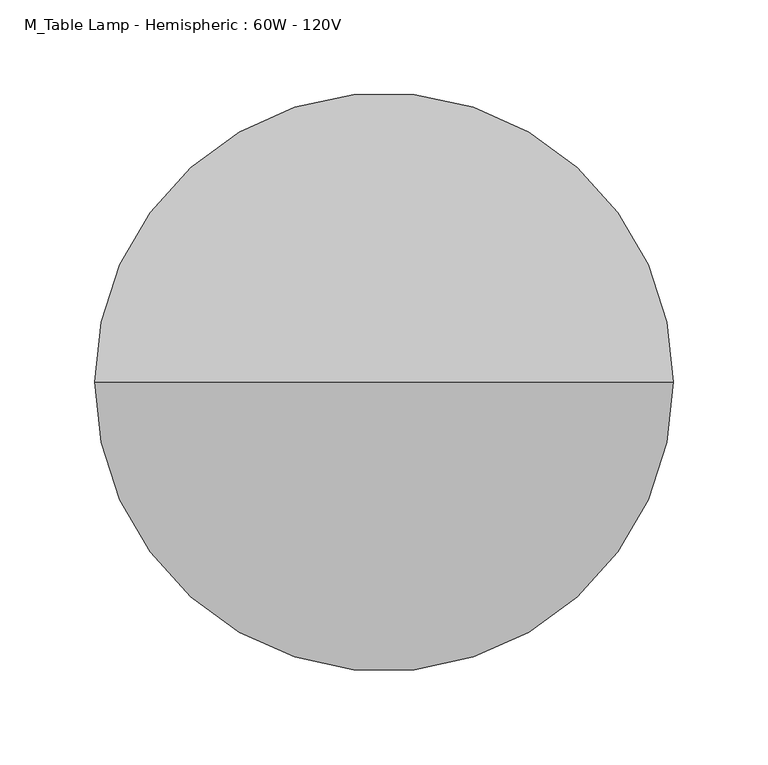
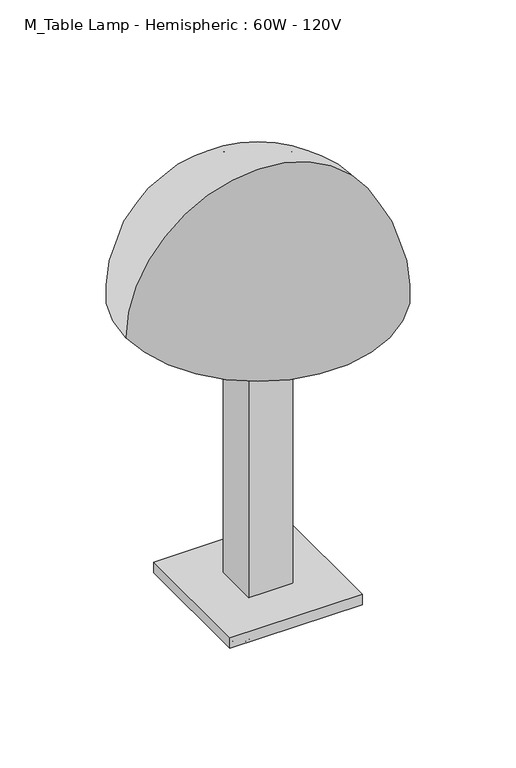
"""IFC4 building model written with IfcOpenShell, lengths in millimetres: light fixture geometry, M_Table Lamp - Hemispheric : 60W - 120V."""

from ifc_helpers import new_model, si_unit, point, frame, origin, origin_2d, place, context, project, spatial, polyline, circle_curve, ellipse_curve, trimmed, segment, composite_curve, outline, extrude, source, transform, mapped, element, save
from ifc_brep_helpers import plane_surface, revolved_surface, advanced_brep


def m_table_lamp_hemispheric_60w_120v_fef6e77c(model_context):
    return source(origin(), model_context, "Body", "SolidModel", [
        extrude(outline(polyline([(76.2, 76.2), (76.2, -76.2), (-76.2, -76.2), (-76.2, 76.2), (76.2, 76.2)])), frame((0.0, 0.0, 12.7), z_axis=(0.0, 0.0, 1.0), x_axis=(1.0, 0.0, 0.0)), (0.0, 0.0, 1.0), 12.7),
        advanced_brep(
        [(34.925, 50.8, 12.7), (66.675, 50.8, 12.7), (53.975, 50.8, 0.0), (47.625, 50.8, 0.0), (47.625, 50.8, 12.7), (53.975, 50.8, 12.7)],
        [
            (0, 1, circle_curve(frame((50.8, 50.8, 12.7), z_axis=(0.0, 0.0, -1.0), x_axis=(1.0, 0.0, 0.0)), 15.875)),
            (1, 2, circle_curve(frame((53.975, 50.8, 12.7), z_axis=(0.0, 1.0, 0.0), x_axis=(1.0, 0.0, 0.0)), 12.7)),
            (2, 3, circle_curve(frame((50.8, 50.8, 0.0), z_axis=(0.0, 0.0, 1.0), x_axis=(1.0, 0.0, 0.0)), 3.175)),
            (3, 0, circle_curve(frame((47.625, 50.8, 12.7), z_axis=(0.0, 1.0, 0.0), x_axis=(-1.0, 0.0, 0.0)), 12.7)),
            (1, 0, circle_curve(frame((50.8, 50.8, 12.7), z_axis=(0.0, 0.0, -1.0), x_axis=(1.0, 0.0, 0.0)), 15.875)),
            (3, 2, circle_curve(frame((50.8, 50.8, 0.0), z_axis=(0.0, 0.0, 1.0), x_axis=(1.0, 0.0, 0.0)), 3.175)),
            (4, 5, circle_curve(frame((50.8, 50.8, 12.7), z_axis=(0.0, 0.0, -1.0), x_axis=(1.0, 0.0, 0.0)), 3.175)),
            (5, 1),
            (0, 4),
            (5, 4, circle_curve(frame((50.8, 50.8, 12.7), z_axis=(0.0, 0.0, -1.0), x_axis=(1.0, 0.0, 0.0)), 3.175)),
            (2, 5),
            (4, 3),
        ],
        [
            revolved_surface(trimmed(ellipse_curve(frame((53.975, 50.8, 12.7), z_axis=(0.0, -1.0, 0.0), x_axis=(1.0, 0.0, 0.0)), 12.7, 12.7), [point((53.975, 50.8, 0.0))], [point((66.675, 50.8, 12.7))], True, "CARTESIAN"), (50.8, 50.8, 36.0623287), (0.0, 0.0, 1.0)),
            plane_surface(frame((50.8, 50.8, 12.7), z_axis=(0.0, 0.0, 1.0), x_axis=(1.0, 0.0, 0.0))),
            revolved_surface(polyline([(53.974999999999994, 50.8, 12.7), (53.974999999999994, 50.8, 0.0)]), (50.8, 50.8, 36.0623287), (0.0, 0.0, 1.0)),
        ],
        [
            (0, [[1, 2, 3, 4]]),
            (0, [[5, -4, 6, -2]]),
            (1, [[7, 8, -1, 9]]),
            (1, [[10, -9, -5, -8]]),
            (2, [[-3, 11, -7, 12]]),
            (2, [[-6, -12, -10, -11]]),
        ],
    ),
        advanced_brep(
        [(34.9494337, -50.8, 12.7), (66.6994337, -50.8, 12.7), (53.9994337, -50.8, 0.0), (47.6494337, -50.8, 0.0), (47.6494337, -50.8, 12.7), (53.9994337, -50.8, 12.7)],
        [
            (0, 1, circle_curve(frame((50.8244337, -50.8, 12.7), z_axis=(0.0, 0.0, -1.0), x_axis=(1.0, 0.0, 0.0)), 15.875)),
            (1, 2, circle_curve(frame((53.9994337, -50.8, 12.7), z_axis=(0.0, 1.0, 0.0), x_axis=(1.0, 0.0, 0.0)), 12.7)),
            (2, 3, circle_curve(frame((50.8244337, -50.8, 0.0), z_axis=(0.0, 0.0, 1.0), x_axis=(1.0, 0.0, 0.0)), 3.175)),
            (3, 0, circle_curve(frame((47.6494337, -50.8, 12.7), z_axis=(0.0, 1.0, 0.0), x_axis=(-1.0, 0.0, 0.0)), 12.7)),
            (1, 0, circle_curve(frame((50.8244337, -50.8, 12.7), z_axis=(0.0, 0.0, -1.0), x_axis=(1.0, 0.0, 0.0)), 15.875)),
            (3, 2, circle_curve(frame((50.8244337, -50.8, 0.0), z_axis=(0.0, 0.0, 1.0), x_axis=(1.0, 0.0, 0.0)), 3.175)),
            (4, 5, circle_curve(frame((50.8244337, -50.8, 12.7), z_axis=(0.0, 0.0, -1.0), x_axis=(1.0, 0.0, 0.0)), 3.175)),
            (5, 1),
            (0, 4),
            (5, 4, circle_curve(frame((50.8244337, -50.8, 12.7), z_axis=(0.0, 0.0, -1.0), x_axis=(1.0, 0.0, 0.0)), 3.175)),
            (2, 5),
            (4, 3),
        ],
        [
            revolved_surface(trimmed(ellipse_curve(frame((53.9994337, -50.8, 12.7), z_axis=(0.0, -1.0, 0.0), x_axis=(1.0, 0.0, 0.0)), 12.7, 12.7), [point((53.9994337, -50.8, 0.0))], [point((66.6994337, -50.8, 12.7))], True, "CARTESIAN"), (50.8244337, -50.8, 36.0623287), (0.0, 0.0, 1.0)),
            plane_surface(frame((50.8244337, -50.8, 12.7), z_axis=(0.0, 0.0, 1.0), x_axis=(1.0, 0.0, 0.0))),
            revolved_surface(polyline([(53.9994337, -50.8, 12.7), (53.9994337, -50.8, 0.0)]), (50.8244337, -50.8, 36.0623287), (0.0, 0.0, 1.0)),
        ],
        [
            (0, [[1, 2, 3, 4]]),
            (0, [[5, -4, 6, -2]]),
            (1, [[7, 8, -1, 9]]),
            (1, [[10, -9, -5, -8]]),
            (2, [[-3, 11, -7, 12]]),
            (2, [[-6, -12, -10, -11]]),
        ],
    ),
        advanced_brep(
        [(-66.7581301, 50.8, 12.7), (-35.0081301, 50.8, 12.7), (-47.7081301, 50.8, 0.0), (-54.0581301, 50.8, 0.0), (-54.0581301, 50.8, 12.7), (-47.7081301, 50.8, 12.7)],
        [
            (0, 1, circle_curve(frame((-50.8831301, 50.8, 12.7), z_axis=(0.0, 0.0, -1.0), x_axis=(1.0, 0.0, 0.0)), 15.875)),
            (1, 2, circle_curve(frame((-47.7081301, 50.8, 12.7), z_axis=(0.0, 1.0, 0.0), x_axis=(1.0, 0.0, 0.0)), 12.7)),
            (2, 3, circle_curve(frame((-50.8831301, 50.8, 0.0), z_axis=(0.0, 0.0, 1.0), x_axis=(1.0, 0.0, 0.0)), 3.175)),
            (3, 0, circle_curve(frame((-54.0581301, 50.8, 12.7), z_axis=(0.0, 1.0, 0.0), x_axis=(-1.0, 0.0, 0.0)), 12.7)),
            (1, 0, circle_curve(frame((-50.8831301, 50.8, 12.7), z_axis=(0.0, 0.0, -1.0), x_axis=(1.0, 0.0, 0.0)), 15.875)),
            (3, 2, circle_curve(frame((-50.8831301, 50.8, 0.0), z_axis=(0.0, 0.0, 1.0), x_axis=(1.0, 0.0, 0.0)), 3.175)),
            (4, 5, circle_curve(frame((-50.8831301, 50.8, 12.7), z_axis=(0.0, 0.0, -1.0), x_axis=(1.0, 0.0, 0.0)), 3.175)),
            (5, 1),
            (0, 4),
            (5, 4, circle_curve(frame((-50.8831301, 50.8, 12.7), z_axis=(0.0, 0.0, -1.0), x_axis=(1.0, 0.0, 0.0)), 3.175)),
            (2, 5),
            (4, 3),
        ],
        [
            revolved_surface(trimmed(ellipse_curve(frame((-47.7081301, 50.8, 12.7), z_axis=(0.0, -1.0, 0.0), x_axis=(1.0, 0.0, 0.0)), 12.7, 12.7), [point((-47.7081301, 50.8, 0.0))], [point((-35.0081301, 50.8, 12.7))], True, "CARTESIAN"), (-50.8831301, 50.8, 36.0623287), (0.0, 0.0, 1.0)),
            plane_surface(frame((-50.8831301, 50.8, 12.7), z_axis=(0.0, 0.0, 1.0), x_axis=(1.0, 0.0, 0.0))),
            revolved_surface(polyline([(-47.708130100000005, 50.8, 12.7), (-47.708130100000005, 50.8, 0.0)]), (-50.8831301, 50.8, 36.0623287), (0.0, 0.0, 1.0)),
        ],
        [
            (0, [[1, 2, 3, 4]]),
            (0, [[5, -4, 6, -2]]),
            (1, [[7, 8, -1, 9]]),
            (1, [[10, -9, -5, -8]]),
            (2, [[-3, 11, -7, 12]]),
            (2, [[-6, -12, -10, -11]]),
        ],
    ),
        advanced_brep(
        [(-66.7336963, -50.8, 12.7), (-34.9836963, -50.8, 12.7), (-47.6836963, -50.8, 0.0), (-54.0336963, -50.8, 0.0), (-54.0336963, -50.8, 12.7), (-47.6836963, -50.8, 12.7)],
        [
            (0, 1, circle_curve(frame((-50.8586963, -50.8, 12.7), z_axis=(0.0, 0.0, -1.0), x_axis=(1.0, 0.0, 0.0)), 15.875)),
            (1, 2, circle_curve(frame((-47.6836963, -50.8, 12.7), z_axis=(0.0, 1.0, 0.0), x_axis=(1.0, 0.0, 0.0)), 12.7)),
            (2, 3, circle_curve(frame((-50.8586963, -50.8, 0.0), z_axis=(0.0, 0.0, 1.0), x_axis=(1.0, 0.0, 0.0)), 3.175)),
            (3, 0, circle_curve(frame((-54.0336963, -50.8, 12.7), z_axis=(0.0, 1.0, 0.0), x_axis=(-1.0, 0.0, 0.0)), 12.7)),
            (1, 0, circle_curve(frame((-50.8586963, -50.8, 12.7), z_axis=(0.0, 0.0, -1.0), x_axis=(1.0, 0.0, 0.0)), 15.875)),
            (3, 2, circle_curve(frame((-50.8586963, -50.8, 0.0), z_axis=(0.0, 0.0, 1.0), x_axis=(1.0, 0.0, 0.0)), 3.175)),
            (4, 5, circle_curve(frame((-50.8586963, -50.8, 12.7), z_axis=(0.0, 0.0, -1.0), x_axis=(1.0, 0.0, 0.0)), 3.175)),
            (5, 1),
            (0, 4),
            (5, 4, circle_curve(frame((-50.8586963, -50.8, 12.7), z_axis=(0.0, 0.0, -1.0), x_axis=(1.0, 0.0, 0.0)), 3.175)),
            (2, 5),
            (4, 3),
        ],
        [
            revolved_surface(trimmed(ellipse_curve(frame((-47.6836963, -50.8, 12.7), z_axis=(0.0, -1.0, 0.0), x_axis=(1.0, 0.0, 0.0)), 12.7, 12.7), [point((-47.6836963, -50.8, 0.0))], [point((-34.9836963, -50.8, 12.7))], True, "CARTESIAN"), (-50.8586963, -50.8, 36.0623287), (0.0, 0.0, 1.0)),
            plane_surface(frame((-50.8586963, -50.8, 12.7), z_axis=(0.0, 0.0, 1.0), x_axis=(1.0, 0.0, 0.0))),
            revolved_surface(polyline([(-47.6836963, -50.8, 12.7), (-47.6836963, -50.8, 0.0)]), (-50.8586963, -50.8, 36.0623287), (0.0, 0.0, 1.0)),
        ],
        [
            (0, [[1, 2, 3, 4]]),
            (0, [[5, -4, 6, -2]]),
            (1, [[7, 8, -1, 9]]),
            (1, [[10, -9, -5, -8]]),
            (2, [[-3, 11, -7, 12]]),
            (2, [[-6, -12, -10, -11]]),
        ],
    ),
        extrude(outline(polyline([(25.4, -25.4), (-25.4, -25.4), (-25.4, 25.4), (25.4, 25.4), (25.4, -25.4)])), frame((0.0, 0.0, 25.4), z_axis=(0.0, 0.0, 1.0), x_axis=(1.0, 0.0, 0.0)), (0.0, 0.0, 1.0), 304.8),
        extrude(outline(composite_curve([segment(trimmed(circle_curve(origin_2d(), 6.35), [point((-6.35, 0.0))], [point((6.35, 0.0))], False, "CARTESIAN"), True, "CONTINUOUS"), segment(trimmed(circle_curve(origin_2d(), 6.35), [point((6.35, 0.0))], [point((-6.35, 0.0))], False, "CARTESIAN"), True, "CONTINUOUS")], self_intersect=False)), frame((0.0, 0.0, 330.2), z_axis=(0.0, 0.0, 1.0), x_axis=(1.0, 0.0, 0.0)), (0.0, 0.0, 1.0), 63.5),
        advanced_brep(
        [(0.0, 0.0, 524.5095504), (152.4, 0.0, 372.1095504), (-152.4, 0.0, 372.1095504), (-146.05, 0.0, 372.1095504), (146.05, 0.0, 372.1095504), (0.0, 0.0, 518.1595504)],
        [
            (0, 1, circle_curve(frame((0.0, 0.0, 372.1095504), z_axis=(0.0, 1.0, 0.0), x_axis=(1.0, 0.0, 0.0)), 152.4)),
            (1, 2, circle_curve(frame((0.0, 0.0, 372.1095504), z_axis=(0.0, 0.0, 1.0), x_axis=(1.0, 0.0, 0.0)), 152.4)),
            (2, 0, circle_curve(frame((0.0, 0.0, 372.1095504), z_axis=(0.0, 1.0, 0.0), x_axis=(-1.0, 0.0, 0.0)), 152.4)),
            (2, 1, circle_curve(frame((0.0, 0.0, 372.1095504), z_axis=(0.0, 0.0, 1.0), x_axis=(1.0, 0.0, 0.0)), 152.4)),
            (3, 4, circle_curve(frame((0.0, 0.0, 372.1095504), z_axis=(0.0, 0.0, -1.0), x_axis=(1.0, 0.0, 0.0)), 146.05)),
            (4, 5, circle_curve(frame((0.0, 0.0, 372.1095504), z_axis=(0.0, -1.0, 0.0), x_axis=(1.0, 0.0, 0.0)), 146.05)),
            (5, 3, circle_curve(frame((0.0, 0.0, 372.1095504), z_axis=(0.0, -1.0, 0.0), x_axis=(-1.0, 0.0, 0.0)), 146.05)),
            (4, 3, circle_curve(frame((0.0, 0.0, 372.1095504), z_axis=(0.0, 0.0, -1.0), x_axis=(1.0, 0.0, 0.0)), 146.05)),
            (1, 4),
            (3, 2),
        ],
        [
            revolved_surface(trimmed(ellipse_curve(frame((0.0, 0.0, 372.1095504), z_axis=(0.0, -1.0, 0.0), x_axis=(1.0, 0.0, 0.0)), 152.4, 152.4), [point((152.4, 0.0, 372.1095504))], [point((0.0, 0.0, 524.5095504))], True, "CARTESIAN"), (0.0, 0.0, 552.6321699), (0.0, 0.0, 1.0)),
            revolved_surface(trimmed(ellipse_curve(frame((0.0, 0.0, 372.1095504), z_axis=(0.0, 1.0, 0.0), x_axis=(1.0, 0.0, 0.0)), 146.05, 146.05), [point((0.0, 0.0, 518.1595504))], [point((146.05, 0.0, 372.1095504))], True, "CARTESIAN"), (0.0, 0.0, 552.6321699), (0.0, 0.0, 1.0)),
            plane_surface(frame((0.0, 0.0, 372.1095504), z_axis=(0.0, 0.0, -1.0), x_axis=(1.0, 0.0, 0.0))),
        ],
        [
            (0, [[1, 2, 3]]),
            (0, [[-3, 4, -1]]),
            (1, [[5, 6, 7]]),
            (1, [[8, -7, -6]]),
            (2, [[-2, 9, -5, 10]]),
            (2, [[-4, -10, -8, -9]]),
        ],
    ),
    ])


if __name__ == "__main__":
    model = new_model("IFC4")
    model_context = context("Model", 3, world=origin())
    ifc_project = project(units=[si_unit("LENGTHUNIT", "METRE", prefix="MILLI")], contexts=[model_context])
    site = spatial("IfcSite", under=ifc_project)
    building = spatial("IfcBuilding", under=site)
    placement = place(None, origin())
    m_table_lamp_hemispheric_60w_120v_shape = m_table_lamp_hemispheric_60w_120v_fef6e77c(model_context)
    element("IfcLightFixture", 1, ObjectType="M_Table Lamp - Hemispheric : 60W - 120V", at=placement, inside=building, context=model_context, shape_type="MappedRepresentation", body=[
        mapped(m_table_lamp_hemispheric_60w_120v_shape, transform((0.0, 0.0, 0.0), x_axis=(1.0, 0.0, 0.0), y_axis=(0.0, 1.0, 0.0), z_axis=(0.0, 0.0, 1.0))),
    ])
    save(model, "model.ifc")

# Revit data of these elements
# Type "M_Table Lamp - Hemispheric : 60W - 120V"
#   Photometric Web File = "TLAE1A19.ies"
#   Assembly Code = "D5020220"
#   Lamp = "A-19"
#   Wattage = 60 W
#   built-in parameter 1150110 = 1 (stored number, unit not read)
#   built-in parameter 1114217 = 1 (stored number, unit not read)
#   built-in parameter 1150109 = 1 (stored number, unit not read)
#   built-in parameter 1150113 = 1 (stored number, unit not read)
#   Tilt Angle = 90.00°
#   built-in parameter 1150115 = 1 (stored number, unit not read)
#   built-in parameter 1150105 = 68.0387 (stored number, unit not read)
#   built-in parameter 1150112 = 1 (stored number, unit not read)
#   built-in parameter 1150114 = 1 (stored number, unit not read)
#   built-in parameter 1150107 = 2800 (stored number, unit not read)
#   built-in parameter 1150106 = 0.680387 (stored number, unit not read)
#   built-in parameter 1150104 = 1.32387 (stored number, unit not read)
#   Voltage = 120 V
#   built-in parameter 1114218 = 1 (stored number, unit not read)
#   built-in parameter 1150133 = 10 (stored number, unit not read)
#   Lumens = 855 lm
#   Apparent Load = 60 VA
#   built-in parameter 1150134 = 4
#   built-in parameter 1150137 = 1
#   Color Filter = 16777215
#   Number of poles = 1
#   Mount Material = Steel, Chrome Plated
#   Shade Material = Plastic, Lamp Shade
#   Base Material = Birch
#   Dimming Lamp Color Temperature Shift = (empty or 0)
#   Default Elevation = 0
#   Wattage Comments = ""
# Element 1 (IfcLightFixture, "M_Table Lamp - Hemispheric : 60W - 120V")
#   Materials on its faces: "Steel, Chrome Plated", "Birch", "Plastic, Lamp Shade"
# Materials
#   "Steel, Chrome Plated": class "Metal", colour RGB 244 244 244, transparency 0, Description = "Chromiuim plated steel", Cost = 0
#   "Plastic, Lamp Shade": class "Glass", colour RGB 250 244 225, transparency 0.58, Description = "physical material", Cost = 0
#   "Birch": class "Wood", colour RGB 224 178 126, transparency 0, Description = "Betula Alleghaniensis", Cost = 0
